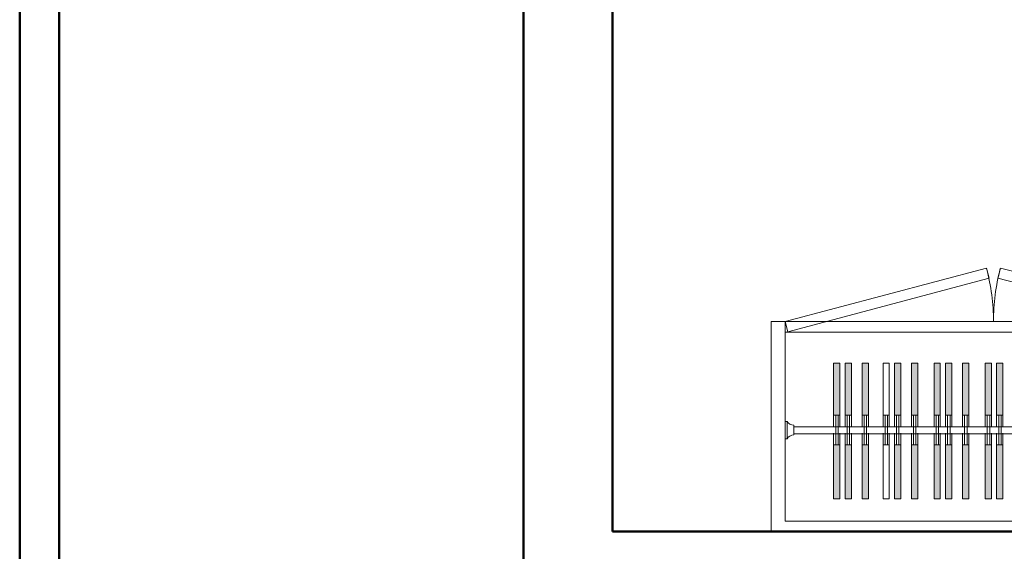
# Model space of a CAD drawing. Units: inches. Extents: x -466983 to 1020, y 324 to 318697.
# Tile 41 of 97: x 392 to 491, y 827 to 881. Entities that reach past the tile are written whole.
import ezdxf

# ---------------------------------------------------------------- set-up
doc = ezdxf.new("R2010")
doc.units = ezdxf.units.IN
doc.header["$MEASUREMENT"] = 0
for name, color, linetype, lineweight in [('A-FLOR-PATT', 252, 'Continuous', 13), ('A-FURN', 8, 'Continuous', 18), ('A-WALL', 7, 'Continuous', 50)]:
    doc.layers.add(name, color=color, linetype=linetype, lineweight=lineweight)

# ---------------------------------------------------------------- blocks, each defined once
blk = doc.blocks.new('Wardrobe')
h = blk.add_hatch(color=256)
h.dxf.hatch_style = 1
h.paths.add_polyline_path([(2766.95, 1539.75), (2766.16, 1539.75), (2766.16, 1532.86), (2766.95, 1532.86)])
h.paths.add_polyline_path([(2766.95, 1529.07), (2766.16, 1529.07), (2766.16, 1522.48), (2766.95, 1522.48)])
h.paths.add_polyline_path([(2799.41, 1529.07), (2798.63, 1529.07), (2798.63, 1522.47), (2799.41, 1522.47)])
h.paths.add_polyline_path([(2799.41, 1539.75), (2798.63, 1539.75), (2798.63, 1532.86), (2799.41, 1532.86)])
h.paths.add_polyline_path([(2813.08, 1539.75), (2812.29, 1539.75), (2812.29, 1532.86), (2813.08, 1532.86)])
h.paths.add_polyline_path([(2813.08, 1529.07), (2812.29, 1529.07), (2812.29, 1522.47), (2813.08, 1522.47)])
h.paths.add_polyline_path([(2825.84, 1539.75), (2825.05, 1539.75), (2825.05, 1532.86), (2825.84, 1532.86)])
h.paths.add_polyline_path([(2825.84, 1529.07), (2825.05, 1529.07), (2825.05, 1522.47), (2825.84, 1522.47)])
h.paths.add_polyline_path([(2782.93, 1539.75), (2782.14, 1539.75), (2782.14, 1532.86), (2782.93, 1532.86)])
h.paths.add_polyline_path([(2782.93, 1529.07), (2782.14, 1529.07), (2782.14, 1522.48), (2782.93, 1522.48)])
h.paths.add_polyline_path([(2838.6, 1539.75), (2837.81, 1539.75), (2837.81, 1532.86), (2838.6, 1532.86)])
h.paths.add_polyline_path([(2838.6, 1529.07), (2837.81, 1529.07), (2837.81, 1522.47), (2838.6, 1522.47)])
h = blk.add_hatch(color=256)
h.dxf.hatch_style = 1
h.paths.add_polyline_path([(2769.11, 1539.75), (2768.32, 1539.75), (2768.32, 1532.86), (2769.11, 1532.86)])
h.paths.add_polyline_path([(2769.11, 1529.07), (2768.32, 1529.07), (2768.32, 1522.48), (2769.11, 1522.48)])
h.paths.add_polyline_path([(2801.57, 1539.75), (2800.79, 1539.75), (2800.79, 1532.86), (2801.57, 1532.86)])
h.paths.add_polyline_path([(2801.57, 1529.07), (2800.79, 1529.07), (2800.79, 1522.47), (2801.57, 1522.47)])
h.paths.add_polyline_path([(2815.24, 1539.75), (2814.45, 1539.75), (2814.45, 1532.86), (2815.24, 1532.86)])
h.paths.add_polyline_path([(2815.24, 1529.07), (2814.45, 1529.07), (2814.45, 1522.47), (2815.24, 1522.47)])
h.paths.add_polyline_path([(2828, 1529.07), (2827.21, 1529.07), (2827.21, 1522.47), (2828, 1522.47)])
h.paths.add_polyline_path([(2828, 1539.75), (2827.21, 1539.75), (2827.21, 1532.86), (2828, 1532.86)])
h.paths.add_polyline_path([(2840.76, 1539.75), (2839.97, 1539.75), (2839.97, 1532.86), (2840.76, 1532.86)])
h.paths.add_polyline_path([(2840.76, 1529.07), (2839.97, 1529.07), (2839.97, 1522.47), (2840.76, 1522.47)])
h.paths.add_polyline_path([(2785.09, 1539.75), (2784.3, 1539.75), (2784.3, 1532.86), (2785.09, 1532.86)])
h.paths.add_polyline_path([(2785.09, 1529.07), (2784.3, 1529.07), (2784.3, 1522.48), (2785.09, 1522.48)])
h = blk.add_hatch(color=256)
h.dxf.hatch_style = 1
h.paths.add_polyline_path([(2770.56, 1539.75), (2769.77, 1539.75), (2769.77, 1532.86), (2770.56, 1532.86)])
h.paths.add_polyline_path([(2770.56, 1529.07), (2769.77, 1529.07), (2769.77, 1522.48), (2770.56, 1522.48)])
h.paths.add_polyline_path([(2786.54, 1539.75), (2785.76, 1539.75), (2785.76, 1532.86), (2786.54, 1532.86)])
h.paths.add_polyline_path([(2786.54, 1529.07), (2785.76, 1529.07), (2785.76, 1522.48), (2786.54, 1522.48)])
h.paths.add_polyline_path([(2803.03, 1539.75), (2802.24, 1539.75), (2802.24, 1532.86), (2803.03, 1532.86)])
h.paths.add_polyline_path([(2803.03, 1529.07), (2802.24, 1529.07), (2802.24, 1522.47), (2803.03, 1522.47)])
h.paths.add_polyline_path([(2816.69, 1539.75), (2815.9, 1539.75), (2815.9, 1532.86), (2816.69, 1532.86)])
h.paths.add_polyline_path([(2816.69, 1529.07), (2815.9, 1529.07), (2815.9, 1522.47), (2816.69, 1522.47)])
h = blk.add_hatch(color=256)
h.dxf.hatch_style = 1
h.paths.add_polyline_path([(2773.22, 1539.75), (2772.43, 1539.75), (2772.43, 1532.86), (2773.22, 1532.86)])
h.paths.add_polyline_path([(2806.16, 1539.75), (2805.37, 1539.75), (2805.37, 1532.86), (2806.16, 1532.86)])
h.paths.add_polyline_path([(2806.16, 1529.07), (2805.37, 1529.07), (2805.37, 1522.47), (2806.16, 1522.47)])
h.paths.add_polyline_path([(2773.22, 1529.07), (2772.43, 1529.07), (2772.43, 1522.48), (2773.22, 1522.48)])
h.paths.add_polyline_path([(2819.35, 1539.75), (2818.56, 1539.75), (2818.56, 1532.86), (2819.35, 1532.86)])
h.paths.add_polyline_path([(2819.35, 1529.07), (2818.56, 1529.07), (2818.56, 1522.47), (2819.35, 1522.47)])
h.paths.add_polyline_path([(2832.33, 1539.75), (2831.54, 1539.75), (2831.54, 1532.86), (2832.33, 1532.86)])
h.paths.add_polyline_path([(2832.33, 1529.07), (2831.54, 1529.07), (2831.54, 1522.47), (2832.33, 1522.47)])
h = blk.add_hatch(color=256)
h.dxf.hatch_style = 1
h.paths.add_polyline_path([(2775.38, 1539.75), (2774.59, 1539.75), (2774.59, 1532.86), (2775.38, 1532.86)])
h.paths.add_polyline_path([(2775.38, 1529.07), (2774.59, 1529.07), (2774.59, 1522.48), (2775.38, 1522.48)])
h.paths.add_polyline_path([(2808.32, 1539.75), (2807.53, 1539.75), (2807.53, 1532.86), (2808.32, 1532.86)])
h.paths.add_polyline_path([(2808.32, 1529.07), (2807.53, 1529.07), (2807.53, 1522.47), (2808.32, 1522.47)])
h.paths.add_polyline_path([(2834.49, 1539.75), (2833.7, 1539.75), (2833.7, 1532.86), (2834.49, 1532.86)])
h.paths.add_polyline_path([(2834.49, 1529.07), (2833.7, 1529.07), (2833.7, 1522.47), (2834.49, 1522.47)])
h = blk.add_hatch(color=256)
h.dxf.hatch_style = 1
h.paths.add_polyline_path([(2776.83, 1539.75), (2776.04, 1539.75), (2776.04, 1532.86), (2776.83, 1532.86)])
h.paths.add_polyline_path([(2776.83, 1529.07), (2776.04, 1529.07), (2776.04, 1522.48), (2776.83, 1522.48)])
h.paths.add_polyline_path([(2809.77, 1539.75), (2808.98, 1539.75), (2808.98, 1532.86), (2809.77, 1532.86)])
h.paths.add_polyline_path([(2809.77, 1529.07), (2808.98, 1529.07), (2808.98, 1522.47), (2809.77, 1522.47)])
h.paths.add_polyline_path([(2821.51, 1539.75), (2820.72, 1539.75), (2820.72, 1532.86), (2821.51, 1532.86)])
h.paths.add_polyline_path([(2821.51, 1529.07), (2820.72, 1529.07), (2820.72, 1522.47), (2821.51, 1522.47)])
h = blk.add_hatch(color=256)
h.dxf.hatch_style = 1
h.paths.add_polyline_path([(2822.96, 1539.75), (2822.17, 1539.75), (2822.17, 1532.86), (2822.96, 1532.86)])
h.paths.add_polyline_path([(2822.96, 1529.07), (2822.17, 1529.07), (2822.17, 1522.47), (2822.96, 1522.47)])
h = blk.add_hatch(color=256)
h.dxf.hatch_style = 1
h.paths.add_polyline_path([(2829.45, 1539.75), (2828.67, 1539.75), (2828.67, 1532.86), (2829.45, 1532.86)])
h.paths.add_polyline_path([(2829.45, 1529.07), (2828.67, 1529.07), (2828.67, 1522.47), (2829.45, 1522.47)])
h.paths.add_polyline_path([(2842.22, 1539.75), (2841.43, 1539.75), (2841.43, 1532.86), (2842.22, 1532.86)])
h.paths.add_polyline_path([(2842.22, 1529.07), (2841.43, 1529.07), (2841.43, 1522.47), (2842.22, 1522.47)])
for p, q in [((2738.89, 1517.19, 0), (2738.89, 1543.9, 0)), ((2738.89, 1543.9, 0), (2850.18, 1543.9, 0)), ((2850.18, 1543.9, 0), (2850.18, 1517.19, 0)), ((2848.4, 1542.57, 0), (2740.67, 1542.57, 0)), ((2740.67, 1542.57, 0), (2740.67, 1517.19, 0)), ((2793.64, 1542.57, 0), (2793.64, 1518.53, 0)), ((2795.43, 1542.57, 0), (2795.43, 1518.53, 0)), ((2848.4, 1517.19, 0), (2848.4, 1542.57, 0)), ((2740.94, 1532.1, 0), (2740.67, 1532.1, 0)), ((2740.94, 1532.1, 0), (2740.67, 1532.1, 0)), ((2740.94, 1532.1, 0), (2740.94, 1529.88, 0)), ((2740.94, 1532.1, 0), (2740.94, 1529.88, 0)), ((2741.78, 1531.61, 0), (2741.78, 1530.37, 0)), ((2741.78, 1531.45, 0), (2792.53, 1531.45, 0)), ((2792.53, 1531.61, 0), (2792.53, 1530.37, 0)), ((2793.38, 1532.1, 0), (2793.38, 1529.88, 0)), ((2793.38, 1532.1, 0), (2793.38, 1529.88, 0)), ((2793.38, 1532.1, 0), (2793.64, 1532.1, 0)), ((2793.38, 1532.1, 0), (2793.64, 1532.1, 0)), ((2795.69, 1532.1, 0), (2795.43, 1532.1, 0)), ((2795.69, 1532.1, 0), (2795.43, 1532.1, 0)), ((2795.69, 1532.1, 0), (2795.69, 1529.88, 0)), ((2795.69, 1532.1, 0), (2795.69, 1529.88, 0)), ((2796.54, 1531.61, 0), (2796.54, 1530.37, 0)), ((2796.54, 1531.45, 0), (2847.29, 1531.45, 0)), ((2847.29, 1531.61, 0), (2847.29, 1530.37, 0)), ((2848.13, 1532.1, 0), (2848.13, 1529.88, 0)), ((2848.13, 1532.1, 0), (2848.13, 1529.88, 0)), ((2848.13, 1532.1, 0), (2848.4, 1532.1, 0)), ((2848.13, 1532.1, 0), (2848.4, 1532.1, 0)), ((2741.78, 1530.56, 0), (2792.53, 1530.56, 0)), ((2796.54, 1530.56, 0), (2847.29, 1530.56, 0)), ((2740.94, 1529.88, 0), (2740.67, 1529.88, 0)), ((2740.94, 1529.88, 0), (2740.67, 1529.88, 0)), ((2793.38, 1529.88, 0), (2793.64, 1529.88, 0)), ((2793.38, 1529.88, 0), (2793.64, 1529.88, 0)), ((2795.69, 1529.88, 0), (2795.43, 1529.88, 0)), ((2795.69, 1529.88, 0), (2795.43, 1529.88, 0)), ((2848.13, 1529.88, 0), (2848.4, 1529.88, 0)), ((2848.13, 1529.88, 0), (2848.4, 1529.88, 0)), ((2848.4, 1518.53, 0), (2740.67, 1518.53, 0)), ((2740.67, 1517.19, 0), (2741.02, 1518.48, 0)), ((2741.02, 1518.48, 0), (2766.6, 1511.65, 0)), ((2794.19, 1518.48, 0), (2767.71, 1511.65, 0)), ((2795.43, 1518.53, 0), (2793.64, 1518.53, 0)), ((2794.53, 1517.19, 0), (2794.19, 1518.48, 0)), ((2794.53, 1517.19, 0), (2794.88, 1518.48, 0)), ((2794.88, 1518.48, 0), (2821.36, 1511.66, 0)), ((2848.05, 1518.48, 0), (2822.47, 1511.66, 0)), ((2848.4, 1517.19, 0), (2848.05, 1518.48, 0)), ((2740.67, 1517.19, 0), (2738.89, 1517.19, 0)), ((2848.4, 1517.19, 0), (2740.67, 1517.19, 0)), ((2766.26, 1510.37, 0), (2740.67, 1517.19, 0)), ((2768.06, 1510.37, 0), (2794.53, 1517.19, 0)), ((2821.01, 1510.37, 0), (2794.53, 1517.19, 0)), ((2822.81, 1510.37, 0), (2848.4, 1517.19, 0)), ((2850.18, 1517.19, 0), (2848.4, 1517.19, 0)), ((2766.6, 1511.65, 0), (2766.26, 1510.37, 0)), ((2767.71, 1511.65, 0), (2768.06, 1510.37, 0)), ((2821.36, 1511.66, 0), (2821.01, 1510.37, 0)), ((2822.47, 1511.66, 0), (2822.81, 1510.37, 0))]:
    blk.add_line(p, q)
at = {"ltscale": 0.106667}
for p, q in [((2745.32, 1522.09, 0), (2763.13, 1539.9, 0)), ((2745.32, 1522.09, 0), (2745.32, 1539.9, 0)), ((2745.32, 1539.9, 0), (2763.13, 1539.9, 0)), ((2763.13, 1522.09, 0), (2745.32, 1539.9, 0)), ((2763.13, 1539.9, 0), (2763.13, 1522.09, 0)), ((2763.13, 1522.09, 0), (2745.32, 1522.09, 0))]:
    blk.add_line(p, q, dxfattribs=at)
at = {"ltscale": 0.037333}
for p, q in [((2766.16, 1531.37, 0), (2766.16, 1539.75, 0)), ((2766.16, 1539.75, 0), (2766.95, 1539.75, 0)), ((2766.95, 1539.75, 0), (2766.95, 1531.37, 0)), ((2768.32, 1531.37, 0), (2768.32, 1539.75, 0)), ((2768.32, 1539.75, 0), (2769.11, 1539.75, 0)), ((2769.11, 1539.75, 0), (2769.11, 1531.37, 0)), ((2769.77, 1531.37, 0), (2769.77, 1539.75, 0)), ((2769.77, 1539.75, 0), (2770.56, 1539.75, 0)), ((2770.56, 1539.75, 0), (2770.56, 1531.37, 0)), ((2772.43, 1531.37, 0), (2772.43, 1539.75, 0)), ((2772.43, 1539.75, 0), (2773.22, 1539.75, 0)), ((2773.22, 1539.75, 0), (2773.22, 1531.37, 0)), ((2774.59, 1531.37, 0), (2774.59, 1539.75, 0)), ((2774.59, 1539.75, 0), (2775.38, 1539.75, 0)), ((2775.38, 1539.75, 0), (2775.38, 1531.37, 0)), ((2776.04, 1531.37, 0), (2776.04, 1539.75, 0)), ((2776.04, 1539.75, 0), (2776.83, 1539.75, 0)), ((2776.83, 1539.75, 0), (2776.83, 1531.37, 0)), ((2782.14, 1531.37, 0), (2782.14, 1539.75, 0)), ((2782.14, 1539.75, 0), (2782.93, 1539.75, 0)), ((2782.93, 1539.75, 0), (2782.93, 1531.37, 0)), ((2784.3, 1531.37, 0), (2784.3, 1539.75, 0)), ((2784.3, 1539.75, 0), (2785.09, 1539.75, 0)), ((2785.09, 1539.75, 0), (2785.09, 1531.37, 0)), ((2785.76, 1531.37, 0), (2785.76, 1539.75, 0)), ((2785.76, 1539.75, 0), (2786.54, 1539.75, 0)), ((2786.54, 1539.75, 0), (2786.54, 1531.37, 0)), ((2798.63, 1531.36, 0), (2798.63, 1539.75, 0)), ((2798.63, 1539.75, 0), (2799.41, 1539.75, 0)), ((2799.41, 1539.75, 0), (2799.41, 1531.36, 0)), ((2800.79, 1531.36, 0), (2800.79, 1539.75, 0)), ((2800.79, 1539.75, 0), (2801.57, 1539.75, 0)), ((2801.57, 1539.75, 0), (2801.57, 1531.36, 0)), ((2802.24, 1531.36, 0), (2802.24, 1539.75, 0)), ((2802.24, 1539.75, 0), (2803.03, 1539.75, 0)), ((2803.03, 1539.75, 0), (2803.03, 1531.36, 0)), ((2805.37, 1531.36, 0), (2805.37, 1539.75, 0)), ((2805.37, 1539.75, 0), (2806.16, 1539.75, 0)), ((2806.16, 1539.75, 0), (2806.16, 1531.36, 0)), ((2807.53, 1531.36, 0), (2807.53, 1539.75, 0)), ((2807.53, 1539.75, 0), (2808.32, 1539.75, 0)), ((2808.32, 1539.75, 0), (2808.32, 1531.36, 0)), ((2808.98, 1531.36, 0), (2808.98, 1539.75, 0)), ((2808.98, 1539.75, 0), (2809.77, 1539.75, 0)), ((2809.77, 1539.75, 0), (2809.77, 1531.36, 0)), ((2812.29, 1531.36, 0), (2812.29, 1539.75, 0)), ((2812.29, 1539.75, 0), (2813.08, 1539.75, 0)), ((2813.08, 1539.75, 0), (2813.08, 1531.36, 0)), ((2814.45, 1531.36, 0), (2814.45, 1539.75, 0)), ((2814.45, 1539.75, 0), (2815.24, 1539.75, 0)), ((2815.24, 1539.75, 0), (2815.24, 1531.36, 0)), ((2815.9, 1531.36, 0), (2815.9, 1539.75, 0)), ((2815.9, 1539.75, 0), (2816.69, 1539.75, 0)), ((2816.69, 1539.75, 0), (2816.69, 1531.36, 0)), ((2818.56, 1531.36, 0), (2818.56, 1539.75, 0)), ((2818.56, 1539.75, 0), (2819.35, 1539.75, 0)), ((2819.35, 1539.75, 0), (2819.35, 1531.36, 0)), ((2820.72, 1531.36, 0), (2820.72, 1539.75, 0)), ((2820.72, 1539.75, 0), (2821.51, 1539.75, 0)), ((2821.51, 1539.75, 0), (2821.51, 1531.36, 0)), ((2822.17, 1531.36, 0), (2822.17, 1539.75, 0)), ((2822.17, 1539.75, 0), (2822.96, 1539.75, 0)), ((2822.96, 1539.75, 0), (2822.96, 1531.36, 0)), ((2825.05, 1531.36, 0), (2825.05, 1539.75, 0)), ((2825.05, 1539.75, 0), (2825.84, 1539.75, 0)), ((2825.84, 1539.75, 0), (2825.84, 1531.36, 0)), ((2827.21, 1531.36, 0), (2827.21, 1539.75, 0)), ((2827.21, 1539.75, 0), (2828, 1539.75, 0)), ((2828, 1539.75, 0), (2828, 1531.36, 0)), ((2828.67, 1531.36, 0), (2828.67, 1539.75, 0)), ((2828.67, 1539.75, 0), (2829.45, 1539.75, 0)), ((2829.45, 1539.75, 0), (2829.45, 1531.36, 0)), ((2831.54, 1531.36, 0), (2831.54, 1539.75, 0)), ((2831.54, 1539.75, 0), (2832.33, 1539.75, 0)), ((2832.33, 1539.75, 0), (2832.33, 1531.36, 0)), ((2833.7, 1531.36, 0), (2833.7, 1539.75, 0)), ((2833.7, 1539.75, 0), (2834.49, 1539.75, 0)), ((2834.49, 1539.75, 0), (2834.49, 1531.36, 0)), ((2835.16, 1531.36, 0), (2835.16, 1539.75, 0)), ((2835.16, 1539.75, 0), (2835.95, 1539.75, 0)), ((2835.95, 1539.75, 0), (2835.95, 1531.36, 0)), ((2837.81, 1531.36, 0), (2837.81, 1539.75, 0)), ((2837.81, 1539.75, 0), (2838.6, 1539.75, 0)), ((2838.6, 1539.75, 0), (2838.6, 1531.36, 0)), ((2839.97, 1531.36, 0), (2839.97, 1539.75, 0)), ((2839.97, 1539.75, 0), (2840.76, 1539.75, 0)), ((2840.76, 1539.75, 0), (2840.76, 1531.36, 0)), ((2841.43, 1531.36, 0), (2841.43, 1539.75, 0)), ((2841.43, 1539.75, 0), (2842.22, 1539.75, 0)), ((2842.22, 1539.75, 0), (2842.22, 1531.36, 0)), ((2766.16, 1532.86, 0), (2766.95, 1532.86, 0)), ((2766.37, 1529.07, 0), (2766.37, 1532.86, 0)), ((2766.69, 1529.07, 0), (2766.69, 1532.86, 0)), ((2768.32, 1532.86, 0), (2769.11, 1532.86, 0)), ((2768.53, 1529.07, 0), (2768.53, 1532.86, 0)), ((2768.84, 1529.07, 0), (2768.84, 1532.86, 0)), ((2769.77, 1532.86, 0), (2770.56, 1532.86, 0)), ((2769.99, 1529.07, 0), (2769.99, 1532.86, 0)), ((2770.3, 1529.07, 0), (2770.3, 1532.86, 0)), ((2772.43, 1532.86, 0), (2773.22, 1532.86, 0)), ((2772.64, 1529.07, 0), (2772.64, 1532.86, 0)), ((2772.96, 1529.07, 0), (2772.96, 1532.86, 0)), ((2774.59, 1532.86, 0), (2775.38, 1532.86, 0)), ((2774.8, 1529.07, 0), (2774.8, 1532.86, 0)), ((2775.11, 1529.07, 0), (2775.11, 1532.86, 0)), ((2776.04, 1532.86, 0), (2776.83, 1532.86, 0)), ((2776.26, 1529.07, 0), (2776.26, 1532.86, 0)), ((2776.57, 1529.07, 0), (2776.57, 1532.86, 0)), ((2782.14, 1532.86, 0), (2782.93, 1532.86, 0)), ((2782.36, 1529.07, 0), (2782.36, 1532.86, 0)), ((2782.67, 1529.07, 0), (2782.67, 1532.86, 0)), ((2784.3, 1532.86, 0), (2785.09, 1532.86, 0)), ((2784.52, 1529.07, 0), (2784.52, 1532.86, 0)), ((2784.83, 1529.07, 0), (2784.83, 1532.86, 0)), ((2785.76, 1532.86, 0), (2786.54, 1532.86, 0)), ((2785.97, 1529.07, 0), (2785.97, 1532.86, 0)), ((2786.28, 1529.07, 0), (2786.28, 1532.86, 0)), ((2798.63, 1532.86, 0), (2799.41, 1532.86, 0)), ((2798.84, 1529.07, 0), (2798.84, 1532.86, 0)), ((2799.15, 1529.07, 0), (2799.15, 1532.86, 0)), ((2800.79, 1532.86, 0), (2801.57, 1532.86, 0)), ((2801, 1529.07, 0), (2801, 1532.86, 0)), ((2801.31, 1529.07, 0), (2801.31, 1532.86, 0)), ((2802.24, 1532.86, 0), (2803.03, 1532.86, 0)), ((2802.45, 1529.07, 0), (2802.45, 1532.86, 0)), ((2802.76, 1529.07, 0), (2802.76, 1532.86, 0)), ((2805.37, 1532.86, 0), (2806.16, 1532.86, 0)), ((2805.58, 1529.07, 0), (2805.58, 1532.86, 0)), ((2805.9, 1529.07, 0), (2805.9, 1532.86, 0)), ((2807.53, 1532.86, 0), (2808.32, 1532.86, 0)), ((2807.74, 1529.07, 0), (2807.74, 1532.86, 0)), ((2808.06, 1529.07, 0), (2808.06, 1532.86, 0)), ((2808.98, 1532.86, 0), (2809.77, 1532.86, 0)), ((2809.2, 1529.07, 0), (2809.2, 1532.86, 0)), ((2809.51, 1529.07, 0), (2809.51, 1532.86, 0)), ((2812.29, 1532.86, 0), (2813.08, 1532.86, 0)), ((2812.51, 1529.07, 0), (2812.51, 1532.86, 0)), ((2812.82, 1529.07, 0), (2812.82, 1532.86, 0)), ((2814.45, 1532.86, 0), (2815.24, 1532.86, 0)), ((2814.67, 1529.07, 0), (2814.67, 1532.86, 0)), ((2814.98, 1529.07, 0), (2814.98, 1532.86, 0)), ((2815.9, 1532.86, 0), (2816.69, 1532.86, 0)), ((2816.12, 1529.07, 0), (2816.12, 1532.86, 0)), ((2816.43, 1529.07, 0), (2816.43, 1532.86, 0)), ((2818.56, 1532.86, 0), (2819.35, 1532.86, 0)), ((2818.78, 1529.07, 0), (2818.78, 1532.86, 0)), ((2819.09, 1529.07, 0), (2819.09, 1532.86, 0)), ((2820.72, 1532.86, 0), (2821.51, 1532.86, 0)), ((2820.94, 1529.07, 0), (2820.94, 1532.86, 0)), ((2821.25, 1529.07, 0), (2821.25, 1532.86, 0)), ((2822.17, 1532.86, 0), (2822.96, 1532.86, 0)), ((2822.39, 1529.07, 0), (2822.39, 1532.86, 0)), ((2822.7, 1529.07, 0), (2822.7, 1532.86, 0)), ((2825.05, 1532.86, 0), (2825.84, 1532.86, 0)), ((2825.27, 1529.07, 0), (2825.27, 1532.86, 0)), ((2825.58, 1529.07, 0), (2825.58, 1532.86, 0)), ((2827.21, 1532.86, 0), (2828, 1532.86, 0)), ((2827.43, 1529.07, 0), (2827.43, 1532.86, 0)), ((2827.74, 1529.07, 0), (2827.74, 1532.86, 0)), ((2828.67, 1532.86, 0), (2829.45, 1532.86, 0)), ((2828.88, 1529.07, 0), (2828.88, 1532.86, 0)), ((2829.19, 1529.07, 0), (2829.19, 1532.86, 0)), ((2831.54, 1532.86, 0), (2832.33, 1532.86, 0)), ((2831.76, 1529.07, 0), (2831.76, 1532.86, 0)), ((2832.07, 1529.07, 0), (2832.07, 1532.86, 0)), ((2833.7, 1532.86, 0), (2834.49, 1532.86, 0)), ((2833.92, 1529.07, 0), (2833.92, 1532.86, 0)), ((2834.23, 1529.07, 0), (2834.23, 1532.86, 0)), ((2835.16, 1532.86, 0), (2835.95, 1532.86, 0)), ((2835.37, 1529.07, 0), (2835.37, 1532.86, 0)), ((2835.68, 1529.07, 0), (2835.68, 1532.86, 0)), ((2837.81, 1532.86, 0), (2838.6, 1532.86, 0)), ((2838.03, 1529.07, 0), (2838.03, 1532.86, 0)), ((2838.34, 1529.07, 0), (2838.34, 1532.86, 0)), ((2839.97, 1532.86, 0), (2840.76, 1532.86, 0)), ((2840.19, 1529.07, 0), (2840.19, 1532.86, 0)), ((2840.5, 1529.07, 0), (2840.5, 1532.86, 0)), ((2841.43, 1532.86, 0), (2842.22, 1532.86, 0)), ((2841.64, 1529.07, 0), (2841.64, 1532.86, 0)), ((2841.95, 1529.07, 0), (2841.95, 1532.86, 0)), ((2766.16, 1522.48, 0), (2766.16, 1530.56, 0)), ((2766.95, 1530.56, 0), (2766.95, 1522.48, 0)), ((2768.32, 1522.48, 0), (2768.32, 1530.56, 0)), ((2769.11, 1530.56, 0), (2769.11, 1522.48, 0)), ((2769.77, 1522.48, 0), (2769.77, 1530.56, 0)), ((2770.56, 1530.56, 0), (2770.56, 1522.48, 0)), ((2772.43, 1522.48, 0), (2772.43, 1530.56, 0)), ((2773.22, 1530.56, 0), (2773.22, 1522.48, 0)), ((2774.59, 1522.48, 0), (2774.59, 1530.56, 0)), ((2775.38, 1530.56, 0), (2775.38, 1522.48, 0)), ((2776.04, 1522.48, 0), (2776.04, 1530.56, 0)), ((2776.83, 1530.56, 0), (2776.83, 1522.48, 0)), ((2782.14, 1522.48, 0), (2782.14, 1530.56, 0)), ((2782.93, 1530.56, 0), (2782.93, 1522.48, 0)), ((2784.3, 1522.48, 0), (2784.3, 1530.56, 0)), ((2785.09, 1530.56, 0), (2785.09, 1522.48, 0)), ((2785.76, 1522.48, 0), (2785.76, 1530.56, 0)), ((2786.54, 1530.56, 0), (2786.54, 1522.48, 0)), ((2798.63, 1522.47, 0), (2798.63, 1530.56, 0)), ((2799.41, 1530.56, 0), (2799.41, 1522.47, 0)), ((2800.79, 1522.47, 0), (2800.79, 1530.56, 0)), ((2801.57, 1530.56, 0), (2801.57, 1522.47, 0)), ((2802.24, 1522.47, 0), (2802.24, 1530.56, 0)), ((2803.03, 1530.56, 0), (2803.03, 1522.47, 0)), ((2805.37, 1522.47, 0), (2805.37, 1530.56, 0)), ((2806.16, 1530.56, 0), (2806.16, 1522.47, 0)), ((2807.53, 1522.47, 0), (2807.53, 1530.56, 0)), ((2808.32, 1530.56, 0), (2808.32, 1522.47, 0)), ((2808.98, 1522.47, 0), (2808.98, 1530.56, 0)), ((2809.77, 1530.56, 0), (2809.77, 1522.47, 0)), ((2812.29, 1522.47, 0), (2812.29, 1530.56, 0)), ((2813.08, 1530.56, 0), (2813.08, 1522.47, 0)), ((2814.45, 1522.47, 0), (2814.45, 1530.56, 0)), ((2815.24, 1530.56, 0), (2815.24, 1522.47, 0)), ((2815.9, 1522.47, 0), (2815.9, 1530.56, 0)), ((2816.69, 1530.56, 0), (2816.69, 1522.47, 0)), ((2818.56, 1522.47, 0), (2818.56, 1530.56, 0)), ((2819.35, 1530.56, 0), (2819.35, 1522.47, 0)), ((2820.72, 1522.47, 0), (2820.72, 1530.56, 0)), ((2821.51, 1530.56, 0), (2821.51, 1522.47, 0)), ((2822.17, 1522.47, 0), (2822.17, 1530.56, 0)), ((2822.96, 1530.56, 0), (2822.96, 1522.47, 0)), ((2825.05, 1522.47, 0), (2825.05, 1530.56, 0)), ((2825.84, 1530.56, 0), (2825.84, 1522.47, 0)), ((2827.21, 1522.47, 0), (2827.21, 1530.56, 0)), ((2828, 1530.56, 0), (2828, 1522.47, 0)), ((2828.67, 1522.47, 0), (2828.67, 1530.56, 0)), ((2829.45, 1530.56, 0), (2829.45, 1522.47, 0)), ((2831.54, 1522.47, 0), (2831.54, 1530.56, 0)), ((2832.33, 1530.56, 0), (2832.33, 1522.47, 0)), ((2833.7, 1522.47, 0), (2833.7, 1530.56, 0)), ((2834.49, 1530.56, 0), (2834.49, 1522.47, 0)), ((2835.16, 1522.47, 0), (2835.16, 1530.56, 0)), ((2835.95, 1530.56, 0), (2835.95, 1522.47, 0)), ((2837.81, 1522.47, 0), (2837.81, 1530.56, 0)), ((2838.6, 1530.56, 0), (2838.6, 1522.47, 0)), ((2839.97, 1522.47, 0), (2839.97, 1530.56, 0)), ((2840.76, 1530.56, 0), (2840.76, 1522.47, 0)), ((2841.43, 1522.47, 0), (2841.43, 1530.56, 0)), ((2842.22, 1530.56, 0), (2842.22, 1522.47, 0)), ((2766.16, 1529.07, 0), (2766.95, 1529.07, 0)), ((2768.32, 1529.07, 0), (2769.11, 1529.07, 0)), ((2769.77, 1529.07, 0), (2770.56, 1529.07, 0)), ((2772.43, 1529.07, 0), (2773.22, 1529.07, 0)), ((2774.59, 1529.07, 0), (2775.38, 1529.07, 0)), ((2776.04, 1529.07, 0), (2776.83, 1529.07, 0)), ((2782.14, 1529.07, 0), (2782.93, 1529.07, 0)), ((2784.3, 1529.07, 0), (2785.09, 1529.07, 0)), ((2785.76, 1529.07, 0), (2786.54, 1529.07, 0)), ((2798.63, 1529.07, 0), (2799.41, 1529.07, 0)), ((2800.79, 1529.07, 0), (2801.57, 1529.07, 0)), ((2802.24, 1529.07, 0), (2803.03, 1529.07, 0)), ((2805.37, 1529.07, 0), (2806.16, 1529.07, 0)), ((2807.53, 1529.07, 0), (2808.32, 1529.07, 0)), ((2808.98, 1529.07, 0), (2809.77, 1529.07, 0)), ((2812.29, 1529.07, 0), (2813.08, 1529.07, 0)), ((2814.45, 1529.07, 0), (2815.24, 1529.07, 0)), ((2815.9, 1529.07, 0), (2816.69, 1529.07, 0)), ((2818.56, 1529.07, 0), (2819.35, 1529.07, 0)), ((2820.72, 1529.07, 0), (2821.51, 1529.07, 0)), ((2822.17, 1529.07, 0), (2822.96, 1529.07, 0)), ((2825.05, 1529.07, 0), (2825.84, 1529.07, 0)), ((2827.21, 1529.07, 0), (2828, 1529.07, 0)), ((2828.67, 1529.07, 0), (2829.45, 1529.07, 0)), ((2831.54, 1529.07, 0), (2832.33, 1529.07, 0)), ((2833.7, 1529.07, 0), (2834.49, 1529.07, 0)), ((2835.16, 1529.07, 0), (2835.95, 1529.07, 0)), ((2837.81, 1529.07, 0), (2838.6, 1529.07, 0)), ((2839.97, 1529.07, 0), (2840.76, 1529.07, 0)), ((2841.43, 1529.07, 0), (2842.22, 1529.07, 0)), ((2766.95, 1522.48, 0), (2766.16, 1522.48, 0)), ((2769.11, 1522.48, 0), (2768.32, 1522.48, 0)), ((2770.56, 1522.48, 0), (2769.77, 1522.48, 0)), ((2773.22, 1522.48, 0), (2772.43, 1522.48, 0)), ((2775.38, 1522.48, 0), (2774.59, 1522.48, 0)), ((2776.83, 1522.48, 0), (2776.04, 1522.48, 0)), ((2782.93, 1522.48, 0), (2782.14, 1522.48, 0)), ((2785.09, 1522.48, 0), (2784.3, 1522.48, 0)), ((2786.54, 1522.48, 0), (2785.76, 1522.48, 0)), ((2799.41, 1522.47, 0), (2798.63, 1522.47, 0)), ((2801.57, 1522.47, 0), (2800.79, 1522.47, 0)), ((2803.03, 1522.47, 0), (2802.24, 1522.47, 0)), ((2806.16, 1522.47, 0), (2805.37, 1522.47, 0)), ((2808.32, 1522.47, 0), (2807.53, 1522.47, 0)), ((2809.77, 1522.47, 0), (2808.98, 1522.47, 0)), ((2813.08, 1522.47, 0), (2812.29, 1522.47, 0)), ((2815.24, 1522.47, 0), (2814.45, 1522.47, 0)), ((2816.69, 1522.47, 0), (2815.9, 1522.47, 0)), ((2819.35, 1522.47, 0), (2818.56, 1522.47, 0)), ((2821.51, 1522.47, 0), (2820.72, 1522.47, 0)), ((2822.96, 1522.47, 0), (2822.17, 1522.47, 0)), ((2825.84, 1522.47, 0), (2825.05, 1522.47, 0)), ((2828, 1522.47, 0), (2827.21, 1522.47, 0)), ((2829.45, 1522.47, 0), (2828.67, 1522.47, 0)), ((2832.33, 1522.47, 0), (2831.54, 1522.47, 0)), ((2834.49, 1522.47, 0), (2833.7, 1522.47, 0)), ((2835.95, 1522.47, 0), (2835.16, 1522.47, 0)), ((2838.6, 1522.47, 0), (2837.81, 1522.47, 0)), ((2840.76, 1522.47, 0), (2839.97, 1522.47, 0)), ((2842.22, 1522.47, 0), (2841.43, 1522.47, 0))]:
    blk.add_line(p, q, dxfattribs=at)
at = {"ltscale": 0.02}
for p, q in [((2742.34, 1537.37, 0), (2742.84, 1537.5, 0)), ((2742.34, 1534.92, 0), (2742.34, 1537.37, 0)), ((2743.67, 1536.85, 0), (2743.67, 1525.18, 0)), ((2740.87, 1534.92, 0), (2740.87, 1535.62, 0)), ((2741.99, 1535.62, 0), (2741.99, 1534.92, 0)), ((2740.67, 1534.92, 0), (2742.84, 1534.92, 0)), ((2742.84, 1534.53, 0), (2740.67, 1534.53, 0)), ((2740.87, 1527.45, 0), (2740.87, 1534.53, 0)), ((2741.99, 1534.53, 0), (2741.99, 1527.45, 0)), ((2742.34, 1527.45, 0), (2742.34, 1534.53, 0)), ((2742.84, 1534.92, 0), (2742.84, 1534.53, 0)), ((2742.84, 1527.45, 0), (2740.67, 1527.45, 0)), ((2740.67, 1527.07, 0), (2742.84, 1527.07, 0)), ((2740.87, 1526.34, 0), (2740.87, 1527.07, 0)), ((2741.99, 1527.07, 0), (2741.99, 1526.34, 0)), ((2742.34, 1524.65, 0), (2742.34, 1527.07, 0)), ((2742.84, 1527.07, 0), (2742.84, 1527.45, 0)), ((2742.86, 1524.53, 0), (2742.34, 1524.65, 0))]:
    blk.add_line(p, q, dxfattribs=at)
for centre, radius, start, end in [((2743.01, 1536.85, 0), 0.668, 360, 104.1887), ((2741.43, 1535.62, 0), 0.556, 0, 180), ((2741.43, 1526.34, 0), 0.556, 180, 0), ((2743.01, 1525.18, 0), 0.668, 257.5257, 0)]:
    blk.add_arc(centre, radius, start, end, dxfattribs=at)
for centre, radius, start, end in [((2741.78, 1532.59, 0), 0.977, 209.9156, 269.9473), ((2741.78, 1532.59, 0), 0.977, 209.9156, 269.9473), ((2792.53, 1532.59, 0), 0.977, 270.0527, 330.0844), ((2792.53, 1532.59, 0), 0.977, 270.0527, 330.0844), ((2796.54, 1532.59, 0), 0.977, 209.9156, 269.9473), ((2796.54, 1532.59, 0), 0.977, 209.9156, 269.9473), ((2847.29, 1532.59, 0), 0.977, 270.0527, 330.0844), ((2847.29, 1532.59, 0), 0.977, 270.0527, 330.0844), ((2741.78, 1529.39, 0), 0.977, 90.0527, 150.0844), ((2792.53, 1529.39, 0), 0.977, 29.9156, 89.9473), ((2796.54, 1529.39, 0), 0.977, 90.0527, 150.0844), ((2847.29, 1529.39, 0), 0.977, 29.9156, 89.9473), ((2740.78, 1517.19, 0), 26.38, 345.1891, 0), ((2793.53, 1517.19, 0), 26.38, 180, 194.8109), ((2795.54, 1517.19, 0), 26.38, 345.1891, 0), ((2848.29, 1517.19, 0), 26.38, 180, 194.8109)]:
    blk.add_arc(centre, radius, start, end)

msp = doc.modelspace()

# ---------------------------------------------------------------- hatches: boundary and pattern name
at = {"layer": 'A-FLOR-PATT', "transparency": 33554572}
h = msp.add_hatch(dxfattribs=at)
h.set_pattern_fill('ANSI37', color=256, scale=30)
h.set_pattern_definition([(45, (-1212.4137, -290.035), (-2.6516504, 2.6516504), []), (135, (-1212.4137, -290.035), (-2.6516504, -2.6516504), [])])
h.paths.add_polyline_path([(901.806, 1075.938), (900.614, 1075.938), (900.614, 1065.386), (899.391, 1065.386), (898.091, 1065.386), (892.836, 1058.71, -0.258377), (892.188, 1058.351), (879.985, 1058.351, -0.20177), (879.438, 1058.581), (874.081, 1065.386), (872.781, 1065.386), (871.558, 1065.386), (871.558, 1075.938), (813.806, 1075.938), (813.806, 1044.792), (832.395, 1044.792, -0.394795), (848.66, 1028.536), (848.66, 1009.938), (901.806, 1009.938), (901.806, 1015.938), (901.306, 1015.938), (871.306, 1015.938), (871.306, 1017.25), (871.334, 1017.25, -0.401453), (901.306, 1045.938), (901.806, 1045.938)])
edge = h.paths.add_edge_path(flags=16)
edge.add_line((847.773, 1068.949), (847.773, 1073.709))
edge.add_arc((849.227, 1073.709), 1.454, 90, 180, ccw=False)
edge.add_line((849.227, 1075.163), (864.492, 1075.163))
edge.add_arc((864.492, 1073.709), 1.454, 0, 90, ccw=False)
edge.add_line((865.946, 1073.709), (865.946, 1069.004))
edge.add_arc((832.645, 1068.976), 33.301, -20.61234, 0.04725, ccw=False)
edge.add_ellipse((856.859, 1058.48), major_axis=(0, 10.213), ratio=0.685919, start_angle=100.00884, end_angle=259.99116, ccw=False)
edge.add_arc((881.074, 1068.976), 33.301, 180.04725, 200.61234, ccw=False)
h.paths.add_polyline_path([(853.146, 1066.482), (853.146, 1066.453), (853.146, 1066.453, 0.433107), (852.917, 1066.685), (852.917, 1066.453), (853.146, 1066.453), (853.146, 1066.482), (853.088, 1066.612, 0.697939), (852.7, 1066.453), (852.7, 1066.453), (852.7, 1066.482), (852.917, 1067.001), (852.917, 1066.685, -0.396254)], flags=0)
h.paths.add_polyline_path([(861.019, 1066.482), (861.019, 1066.453), (861.019, 1066.453, 0.416404), (860.802, 1066.685), (860.802, 1066.453), (861.019, 1066.453), (861.019, 1066.482), (860.967, 1066.605, 0.713344), (860.573, 1066.453), (860.573, 1066.453), (860.573, 1066.482), (860.802, 1067.001), (860.802, 1066.685, -0.379973)], flags=0)
edge = h.paths.add_edge_path(flags=0)
edge.add_spline(control_points=[(861.13, 1065.785), (861.466, 1065.248), (861.613, 1065.016), (861.983, 1064.374), (862.192, 1063.944), (862.561, 1063.039), (862.721, 1062.563), (862.987, 1061.578), (863.092, 1061.069), (863.245, 1060.031), (863.293, 1059.503), (863.329, 1058.441), (863.318, 1057.908), (863.237, 1056.852), (863.166, 1056.329), (862.97, 1055.308), (862.843, 1054.81), (862.537, 1053.852), (862.357, 1053.393), (861.951, 1052.525), (861.725, 1052.117), (861.233, 1051.362), (860.967, 1051.016), (860.405, 1050.395), (860.108, 1050.12), (859.494, 1049.646), (859.176, 1049.448), (858.528, 1049.13), (858.197, 1049.011), (857.531, 1048.852), (857.196, 1048.812), (856.525, 1048.812), (856.189, 1048.852), (855.524, 1049.01), (855.193, 1049.129), (854.545, 1049.447), (854.227, 1049.645), (853.612, 1050.118), (853.316, 1050.393), (852.753, 1051.014), (852.487, 1051.36), (851.995, 1052.114), (851.769, 1052.523), (851.363, 1053.39), (851.183, 1053.85), (850.877, 1054.807), (850.75, 1055.305), (850.553, 1056.326), (850.483, 1056.849), (850.401, 1057.905), (850.39, 1058.438), (850.426, 1059.5), (850.473, 1060.028), (850.626, 1061.066), (850.732, 1061.575), (850.997, 1062.561), (851.157, 1063.036), (851.525, 1063.942), (851.734, 1064.371), (852.106, 1065.016), (852.254, 1065.25), (852.608, 1065.733)], knot_values=[3.915332, 3.915332, 3.915332, 3.915332, 4.013468, 4.013468, 4.175532, 4.175532, 4.337596, 4.337596, 4.49966, 4.49966, 4.661724, 4.661724, 4.823788, 4.823788, 4.985852, 4.985852, 5.147916, 5.147916, 5.30998, 5.30998, 5.472044, 5.472044, 5.634109, 5.634109, 5.796173, 5.796173, 5.958237, 5.958237, 6.120301, 6.120301, 6.282365, 6.282365, 6.444429, 6.444429, 6.606493, 6.606493, 6.768557, 6.768557, 6.930621, 6.930621, 7.092685, 7.092685, 7.254749, 7.254749, 7.416813, 7.416813, 7.578878, 7.578878, 7.740942, 7.740942, 7.903006, 7.903006, 8.06507, 8.06507, 8.227134, 8.227134, 8.389198, 8.389198, 8.551262, 8.551262, 8.65037, 8.65037, 8.65037, 8.65037], degree=3, periodic=0)
edge.add_line((852.642, 1065.785), (861.13, 1065.785))
edge = h.paths.add_edge_path(flags=0)
edge.add_ellipse((856.85, 1057.743), major_axis=(0, 7.792), ratio=0.687861, start_angle=0, end_angle=360)
h.paths.add_polyline_path([(848.863, 1069.389), (848.863, 1073.96, -0.414214), (849.954, 1075.051), (863.765, 1075.051, -0.414214), (864.856, 1073.96), (864.856, 1069.389, -0.388936), (864.524, 1069.027, -0.043561), (849.195, 1069.027, -0.388936)], flags=0)
h.paths.add_polyline_path([(853.101, 1068.112, -1), (852.677, 1068.112, -1)], flags=0)
edge = h.paths.add_edge_path(flags=0)
edge.add_ellipse((856.859, 1057.338), major_axis=(0, 2.207), ratio=0.657164, start_angle=0, end_angle=360)
h.paths.add_polyline_path([(861.041, 1068.112, -1), (860.618, 1068.112, -1)], flags=0)
edge = h.paths.add_edge_path()
edge.add_line((573.954, 1057.341), (573.954, 1075.938))
edge.add_line((573.954, 1075.938), (558.731, 1075.938))
edge.add_line((558.731, 1075.938), (558.731, 1065.386))
edge.add_line((558.731, 1065.386), (557.507, 1065.386))
edge.add_line((557.507, 1065.386), (556.207, 1065.386))
edge.add_line((556.207, 1065.386), (550.952, 1058.71))
edge.add_arc((550.304, 1059.116), 0.765, 270, 327.94832, ccw=False)
edge.add_line((550.304, 1058.351), (538.101, 1058.351))
edge.add_arc((538.101, 1059.116), 0.765, 224.3704, 270, ccw=False)
edge.add_line((537.555, 1058.581), (532.198, 1065.386))
edge.add_line((532.198, 1065.386), (530.898, 1065.386))
edge.add_line((530.898, 1065.386), (529.674, 1065.386))
edge.add_line((529.674, 1065.386), (529.674, 1075.938))
edge.add_line((529.674, 1075.938), (520.806, 1075.938))
edge.add_line((520.806, 1075.938), (520.806, 1045.938))
edge.add_line((520.806, 1045.938), (521.306, 1045.938))
edge.add_arc((521.306, 1015.938), 30, 2.50749, 90, ccw=False)
edge.add_line((551.277, 1017.25), (551.306, 1017.25))
edge.add_line((551.306, 1017.25), (551.306, 1015.938))
edge.add_line((551.306, 1015.938), (520.806, 1015.938))
edge.add_line((520.806, 1015.938), (520.806, 1009.938))
edge.add_line((520.806, 1009.938), (559.191, 1010.402))
edge.add_arc((559.191, 1011.856), 1.454, 180, 270, ccw=False)
edge.add_line((557.737, 1011.856), (557.737, 1016.561))
edge.add_arc((591.039, 1016.589), 33.301, 159.38766, 180.04725, ccw=False)
edge.add_ellipse((566.824, 1027.085), major_axis=(0, 10.213), ratio=0.685919, start_angle=280.00884, end_angle=439.99116, ccw=False)
edge.add_arc((542.609, 1016.589), 33.301, 0.04725, 20.61234, ccw=False)
edge.add_line((575.91, 1016.616), (575.91, 1011.856))
edge.add_arc((574.456, 1011.856), 1.454, -90, 0, ccw=False)
edge.add_line((574.456, 1010.402), (608.806, 1009.938))
edge.add_line((608.806, 1009.938), (608.806, 1041.086))
edge.add_line((608.806, 1041.086), (590.218, 1041.086))
edge.add_arc((590.775, 1057.907), 16.831, 181.92775, 268.10321, ccw=False)
edge = h.paths.add_edge_path()
edge.add_ellipse((494.244, 583.62), major_axis=(0, 10.213), ratio=0.685919, start_angle=280.00884, end_angle=439.99116, ccw=False)
edge.add_arc((470.03, 573.124), 33.301, 0.04725, 20.61234, ccw=False)
edge.add_line((503.331, 573.152), (503.331, 568.392))
edge.add_arc((501.877, 568.392), 1.454, -90, 0, ccw=False)
edge.add_line((501.877, 566.938), (539.806, 566.938))
edge.add_line((539.806, 566.938), (539.806, 572.938))
edge.add_line((539.806, 572.938), (539.306, 572.938))
edge.add_line((539.306, 572.938), (509.306, 572.938))
edge.add_line((509.306, 572.938), (509.306, 574.25))
edge.add_line((509.306, 574.25), (509.334, 574.25))
edge.add_arc((539.306, 572.938), 30, 90, 177.49251, ccw=False)
edge.add_line((539.306, 602.938), (539.806, 602.938))
edge.add_line((539.806, 602.938), (539.806, 626.938))
edge.add_line((539.806, 626.938), (531.772, 626.938))
edge.add_line((531.772, 626.938), (531.772, 616.386))
edge.add_line((531.772, 616.386), (530.548, 616.386))
edge.add_line((530.548, 616.386), (529.249, 616.386))
edge.add_line((529.249, 616.386), (523.711, 609.351))
edge.add_line((523.711, 609.351), (510.777, 609.351))
edge.add_line((510.777, 609.351), (505.239, 616.386))
edge.add_line((505.239, 616.386), (503.939, 616.386))
edge.add_line((503.939, 616.386), (502.715, 616.386))
edge.add_line((502.715, 616.386), (502.715, 626.938))
edge.add_line((502.715, 626.938), (481.698, 626.938))
edge.add_line((481.698, 626.938), (481.698, 610.995))
edge.add_arc((467.27, 611.473), 14.436, 271.92775, 358.10321, ccw=False)
edge.add_line((467.756, 597.045), (451.806, 597.045))
edge.add_line((451.806, 597.045), (451.806, 584.404))
edge.add_line((451.806, 584.404), (451.806, 566.938))
edge.add_line((451.806, 566.938), (486.612, 566.938))
edge.add_arc((486.612, 568.392), 1.454, 180, 270, ccw=False)
edge.add_line((485.158, 568.392), (485.158, 573.097))
edge.add_arc((518.459, 573.124), 33.301, 159.38766, 180.04725, ccw=False)
h.paths.add_polyline_path([(836.261, 1020.733), (879.89, 1020.733), (879.89, 1039.39), (836.261, 1039.39)], flags=25)
h.paths.add_polyline_path([(549.985, 1036.749), (593.614, 1036.749), (593.614, 1055.407), (549.985, 1055.407)], flags=24)
h.paths.add_polyline_path([(475.123, 595.596), (518.752, 595.596), (518.752, 614.253), (475.123, 614.253)], flags=24)

# ---------------------------------------------------------------- linework, layer by layer
at = {"layer": 'A-WALL'}
for p, q in [((391.806, 364.938), (391.806, 1084.938)), ((442.806, 415.938), (442.806, 1084.938)), ((395.806, 368.938), (395.806, 1080.938)), ((451.806, 828.938), (451.806, 1075.938)), ((608.806, 828.938), (451.806, 828.938))]:
    msp.add_line(p, q, dxfattribs=at)

# ---------------------------------------------------------------- block references
at = {"layer": 'A-FURN', "xscale": 0.7967580954171016, "yscale": 0.7967580954171016, "zscale": 0.7967580954171016, "rotation": 180}
msp.add_blockref('Wardrobe', (2738.768, 2059.054), dxfattribs=at)

doc.saveas('drawing.dxf')
